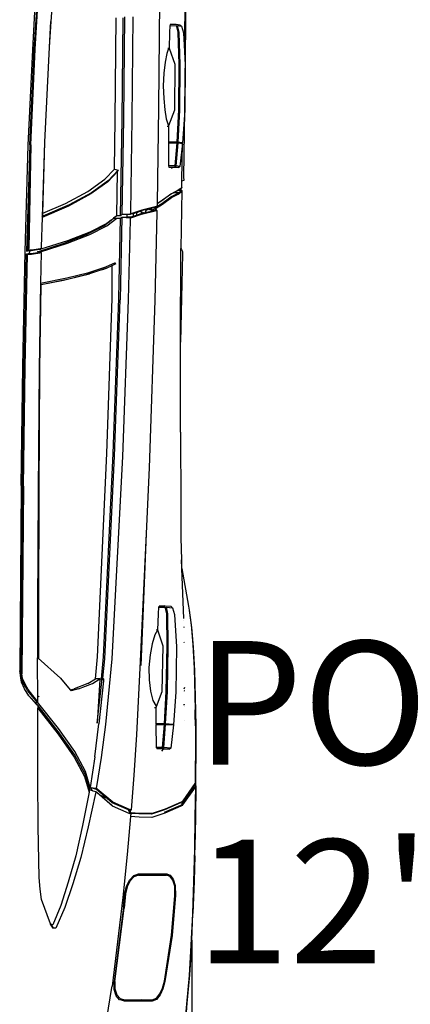
# Model space of a CAD drawing. Units: inches. Extents: x -4737294 to -4736756, y 1716389 to 1717040.
# Tile 10 of 25: x -4737123 to -4737096, y 1716491 to 1716559. Entities that reach past the tile are written whole.
import ezdxf

# ---------------------------------------------------------------- set-up
doc = ezdxf.new("R2010")
doc.units = ezdxf.units.IN
doc.header["$MEASUREMENT"] = 0
doc.layers.add('A-AREA-IDEN', color=250, linetype='Continuous', lineweight=18)
doc.layers.add('A-EQPM-VEHI', color=250, linetype='Continuous', lineweight=13)
doc.layers.add('Edges', color=250, linetype='Continuous')
doc.styles.get("Standard").update_dxf_attribs({"font": 'arial.ttf'})

# ---------------------------------------------------------------- blocks, each defined once
blk = doc.blocks.new('Nissan Qashqai pl')
at = {"layer": 'Edges'}
for p, q in [((10.4889, 12.8119), (10.526, 12.8138)), ((10.4926, 12.8125), (10.5294, 12.8143)), ((10.526, 12.8138), (10.569, 12.8151)), ((10.5294, 12.8143), (10.5719, 12.8156)), ((10.569, 12.8151), (10.5919, 12.8155)), ((10.5719, 12.8156), (10.6176, 12.8164)), ((10.5919, 12.8155), (10.6151, 12.8159)), ((10.5981, 12.8157), (10.5919, 12.8155)), ((10.6174, 12.816), (10.5981, 12.8157)), ((10.6151, 12.8159), (10.6644, 12.8162)), ((10.6176, 12.8164), (10.6651, 12.8167)), ((10.6644, 12.8162), (10.7078, 12.8159)), ((10.6651, 12.8167), (10.666, 12.8167)), ((10.666, 12.8167), (10.677, 12.8167)), ((10.6729, 12.8157), (10.7082, 12.8156)), ((10.6809, 12.8167), (10.677, 12.8167)), ((10.7128, 12.8166), (10.6809, 12.8167)), ((10.7078, 12.8159), (10.7083, 12.8156)), ((10.7082, 12.8156), (10.7078, 12.8159)), ((10.7085, 12.8153), (10.7082, 12.8156)), ((10.7082, 12.8156), (10.7083, 12.8156)), ((10.7083, 12.8156), (10.7087, 12.8153)), ((10.7083, 12.8156), (10.7125, 12.8156)), ((10.7087, 12.8153), (10.7363, 12.7959)), ((10.7139, 12.8164), (10.7125, 12.8156)), ((10.7137, 12.8148), (10.7125, 12.8156)), ((10.7128, 12.8166), (10.7625, 12.8161)), ((10.7128, 12.8166), (10.724, 12.8166)), ((10.7137, 12.8148), (10.7138, 12.8147)), ((10.7418, 12.7947), (10.7138, 12.8147)), ((10.7139, 12.8164), (10.7148, 12.8157)), ((10.7628, 12.8158), (10.7139, 12.8164)), ((10.7148, 12.8157), (10.7429, 12.7956)), ((10.7685, 12.8161), (10.724, 12.8166)), ((10.7625, 12.8161), (10.7628, 12.8161)), ((10.7628, 12.8161), (10.8099, 12.8152)), ((10.8131, 12.8149), (10.7628, 12.8158)), ((10.7688, 12.8161), (10.7685, 12.8161)), ((10.8099, 12.8152), (10.7688, 12.8161)), ((10.8099, 12.8152), (10.8131, 12.8152)), ((10.8134, 12.8152), (10.8131, 12.8152)), ((10.8644, 12.8135), (10.8131, 12.8149)), ((10.8134, 12.8152), (10.8142, 12.8152)), ((10.8142, 12.8152), (10.8142, 12.8152)), ((10.8237, 12.8149), (10.8142, 12.8152)), ((10.8237, 12.8149), (10.864, 12.8138)), ((10.8596, 12.8138), (10.8589, 12.8138)), ((10.8642, 12.8136), (10.8596, 12.8138)), ((10.864, 12.8138), (10.8642, 12.8138)), ((10.8642, 12.8138), (10.9152, 12.812)), ((9.2517, 12.8031), (9.5372, 12.7983)), ((9.641, 12.7991), (9.351, 12.803)), ((9.5176, 12.7972), (9.5372, 12.7983)), ((9.5372, 12.7983), (9.5689, 12.7999)), ((9.5689, 12.7999), (9.641, 12.7991)), ((9.641, 12.7991), (9.6921, 12.7956)), ((9.7466, 12.7978), (9.641, 12.7991)), ((10.3679, 12.7944), (10.4275, 12.8051)), ((10.4275, 12.8051), (10.4304, 12.8056)), ((10.4304, 12.8056), (10.4339, 12.8061)), ((10.4339, 12.8061), (10.4573, 12.8093)), ((10.4339, 12.8061), (10.4345, 12.8062)), ((10.4345, 12.8062), (10.4613, 12.8099)), ((10.4573, 12.8093), (10.4889, 12.8119)), ((10.4613, 12.8099), (10.4926, 12.8125)), ((10.4838, 12.7977), (10.4852, 12.7982)), ((10.5565, 12.7985), (10.5591, 12.7977)), ((10.5615, 12.7978), (10.5617, 12.7985)), ((10.583, 12.7984), (10.5834, 12.798)), ((10.5836, 12.798), (10.5831, 12.7984)), ((10.5847, 12.798), (10.5841, 12.7984)), ((10.5873, 12.7981), (10.5873, 12.7981)), ((10.6087, 12.7983), (10.6087, 12.7984)), ((10.9158, 12.8118), (10.8644, 12.8135)), ((10.9577, 12.8101), (10.9152, 12.812)), ((10.9657, 12.8095), (10.9158, 12.8118)), ((10.9577, 12.8101), (10.9649, 12.8097)), ((10.9577, 12.8101), (11.1283, 12.8101)), ((10.9649, 12.8097), (11.0127, 12.8067)), ((11.0138, 12.8064), (10.9657, 12.8095)), ((11.0127, 12.8067), (11.0576, 12.8026)), ((11.059, 12.8023), (11.0138, 12.8064)), ((11.0576, 12.8026), (11.0798, 12.8008)), ((11.0768, 12.8008), (11.059, 12.8023)), ((9.5052, 12.7918), (9.5044, 12.7856)), ((9.5044, 12.7856), (9.5045, 12.7814)), ((9.5052, 12.7918), (9.5069, 12.7941)), ((9.5061, 12.7878), (9.5069, 12.7941)), ((9.5168, 12.7904), (9.5061, 12.7878)), ((9.5061, 12.7856), (9.5167, 12.7883)), ((9.5063, 12.7755), (9.5061, 12.7856)), ((9.5069, 12.7941), (9.5176, 12.7972)), ((9.5167, 12.7883), (9.5679, 12.7899)), ((9.5679, 12.792), (9.5168, 12.7904)), ((9.5678, 12.7837), (9.5426, 12.7747)), ((9.64, 12.7831), (9.5678, 12.7837)), ((9.6401, 12.7914), (9.5679, 12.792)), ((9.5679, 12.7899), (9.64, 12.7892)), ((9.64, 12.7892), (9.6912, 12.7865)), ((9.6645, 12.7737), (9.64, 12.7831)), ((9.6913, 12.7886), (9.6401, 12.7914)), ((9.6913, 12.7886), (9.6912, 12.7865)), ((9.6912, 12.7865), (9.6912, 12.7811)), ((9.692, 12.7943), (9.6913, 12.7886)), ((9.6921, 12.7956), (9.692, 12.7943)), ((9.6922, 12.7943), (9.692, 12.7943)), ((9.692, 12.7811), (9.6921, 12.7864)), ((9.6922, 12.7943), (9.6921, 12.7956)), ((9.7526, 12.7946), (9.6921, 12.7956)), ((9.6922, 12.7885), (9.6921, 12.7864)), ((9.6921, 12.7864), (9.7288, 12.7832)), ((9.6922, 12.7885), (9.693, 12.7955)), ((9.6922, 12.7885), (9.6922, 12.7943)), ((9.7288, 12.7854), (9.6922, 12.7885)), ((9.693, 12.7955), (9.7296, 12.7914)), ((9.7288, 12.7832), (9.7287, 12.7734)), ((9.7296, 12.7914), (9.7288, 12.7854)), ((9.7306, 12.7834), (9.7288, 12.7854)), ((9.7288, 12.7854), (9.7288, 12.7832)), ((9.7288, 12.7832), (9.7306, 12.7834)), ((9.7296, 12.7914), (9.7314, 12.7895)), ((9.7305, 12.7738), (9.7306, 12.7834)), ((9.7306, 12.7834), (9.7314, 12.7895)), ((9.7314, 12.7895), (9.7313, 12.7798)), ((9.7511, 12.7979), (9.7466, 12.7978)), ((9.7526, 12.7946), (9.7511, 12.7979)), ((9.7623, 12.7945), (9.7526, 12.7946)), ((9.7623, 12.7945), (9.7643, 12.7937)), ((9.7643, 12.7937), (9.7652, 12.7927)), ((9.7643, 12.7937), (9.7648, 12.7929)), ((9.7648, 12.7929), (9.7648, 12.7929)), ((9.7648, 12.7929), (9.7664, 12.7902)), ((9.7652, 12.7927), (9.7665, 12.7907)), ((9.7665, 12.7904), (9.7664, 12.7902)), ((9.7664, 12.7902), (9.7674, 12.7885)), ((9.7667, 12.7933), (9.7665, 12.7907)), ((9.7665, 12.7907), (9.7676, 12.7889)), ((9.7677, 12.7944), (9.7667, 12.7933)), ((9.7676, 12.7931), (9.7667, 12.7933)), ((9.7673, 12.7899), (9.7676, 12.7931)), ((9.7673, 12.7897), (9.7673, 12.7899)), ((9.7673, 12.7897), (9.7676, 12.7889)), ((9.7674, 12.7885), (9.7728, 12.7781)), ((9.769, 12.7926), (9.7676, 12.7931)), ((9.7676, 12.7889), (9.7684, 12.7875)), ((9.7676, 12.7887), (9.7678, 12.7882)), ((9.7677, 12.7944), (9.7677, 12.7944)), ((9.77, 12.7936), (9.7677, 12.7944)), ((9.7677, 12.7944), (9.8598, 12.7928)), ((9.7684, 12.7875), (9.7717, 12.781)), ((9.7712, 12.7892), (9.769, 12.7926)), ((9.7734, 12.7884), (9.77, 12.7936)), ((9.7707, 12.7848), (9.7709, 12.7893)), ((9.7717, 12.781), (9.7707, 12.7848)), ((9.7709, 12.7893), (9.7712, 12.7892)), ((9.7724, 12.7874), (9.7712, 12.7892)), ((9.7778, 12.777), (9.7724, 12.7874)), ((9.7788, 12.778), (9.7734, 12.7884)), ((9.8598, 12.7928), (9.8614, 12.7937)), ((9.8643, 12.7927), (9.8598, 12.7928)), ((9.8614, 12.7937), (9.8647, 12.7956)), ((10.0085, 12.7922), (9.8643, 12.7927)), ((9.8647, 12.7956), (9.869, 12.7954)), ((9.869, 12.7954), (10.0085, 12.7922)), ((10.0124, 12.7922), (10.0085, 12.7922)), ((10.1513, 12.7924), (10.0124, 12.7922)), ((10.1513, 12.7924), (10.2677, 12.793)), ((10.2677, 12.793), (10.3189, 12.7931)), ((10.3189, 12.7931), (10.3537, 12.7939)), ((10.3537, 12.7939), (10.3832, 12.7945)), ((10.3679, 12.7944), (10.3537, 12.7939)), ((10.4468, 12.7976), (10.3679, 12.7944)), ((10.4299, 12.7798), (10.4406, 12.7829)), ((10.4406, 12.7829), (10.4919, 12.7858)), ((10.4503, 12.7976), (10.4502, 12.7976)), ((10.4603, 12.7976), (10.4613, 12.7978)), ((10.4919, 12.7858), (10.564, 12.7851)), ((10.564, 12.7851), (10.6151, 12.7813)), ((10.7363, 12.7959), (10.7376, 12.795)), ((10.7387, 12.794), (10.7376, 12.795)), ((10.7376, 12.795), (10.7378, 12.7946)), ((10.7378, 12.7946), (10.7379, 12.7945)), ((10.7378, 12.7946), (10.7385, 12.7932)), ((10.7385, 12.7932), (10.7497, 12.7679)), ((10.7387, 12.794), (10.7396, 12.7922)), ((10.7396, 12.7922), (10.7507, 12.7669)), ((10.743, 12.7939), (10.7418, 12.7947)), ((10.7432, 12.7954), (10.7426, 12.7954)), ((10.7429, 12.7956), (10.7432, 12.7954)), ((10.7434, 12.793), (10.743, 12.7939)), ((10.7441, 12.7954), (10.7432, 12.7954)), ((10.7432, 12.7954), (10.744, 12.7948)), ((10.7437, 12.7921), (10.7434, 12.793)), ((10.7438, 12.7921), (10.7437, 12.7921)), ((10.7438, 12.7921), (10.7549, 12.7666)), ((10.744, 12.7948), (10.7448, 12.793)), ((10.7448, 12.793), (10.7559, 12.7674)), ((10.8607, 12.7808), (10.8708, 12.7841)), ((10.8716, 12.7832), (10.8622, 12.7801)), ((10.8708, 12.7841), (10.8869, 12.7844)), ((10.887, 12.7835), (10.8716, 12.7832)), ((10.8869, 12.7844), (10.9499, 12.7789)), ((10.9498, 12.7781), (10.887, 12.7835)), ((9.5037, 12.7806), (9.5045, 12.7814)), ((9.5045, 12.7814), (9.5045, 12.7759)), ((9.5045, 12.7759), (9.5063, 12.7755)), ((9.5063, 12.7755), (9.5168, 12.7751)), ((9.5168, 12.7751), (9.5423, 12.7746)), ((9.5423, 12.7746), (9.5422, 12.7736)), ((9.5422, 12.7736), (9.5422, 12.7725)), ((9.5422, 12.7736), (9.5424, 12.7735)), ((9.5426, 12.7747), (9.5423, 12.7746)), ((9.5426, 12.7747), (9.5424, 12.7735)), ((9.5424, 12.7735), (9.5503, 12.7706)), ((9.5503, 12.7706), (9.5641, 12.7681)), ((9.5641, 12.7681), (9.5818, 12.766)), ((9.6215, 12.766), (9.6395, 12.7676)), ((9.6395, 12.7676), (9.654, 12.7697)), ((9.654, 12.7697), (9.6633, 12.7726)), ((9.6633, 12.7726), (9.6645, 12.7737)), ((9.6655, 12.7733), (9.6645, 12.7737)), ((9.6655, 12.7733), (9.6911, 12.7732)), ((9.6655, 12.7713), (9.6655, 12.7733)), ((9.6912, 12.7811), (9.6911, 12.7796)), ((9.6911, 12.7796), (9.6911, 12.7732)), ((9.6911, 12.7732), (9.692, 12.7733)), ((9.692, 12.7811), (9.6912, 12.7811)), ((9.692, 12.7796), (9.692, 12.7811)), ((9.692, 12.7733), (9.692, 12.7796)), ((9.692, 12.7733), (9.7287, 12.7734)), ((9.7287, 12.7734), (9.7305, 12.7738)), ((9.7305, 12.7738), (9.7313, 12.7798)), ((9.733, 12.7782), (9.7313, 12.7798)), ((9.7717, 12.781), (9.7738, 12.7771)), ((9.7728, 12.7781), (9.7832, 12.7637)), ((9.7738, 12.7771), (9.7842, 12.7627)), ((9.7883, 12.7626), (9.7778, 12.777)), ((9.7894, 12.7636), (9.7788, 12.778)), ((10.4263, 12.7665), (10.4274, 12.7674)), ((10.4282, 12.7775), (10.4274, 12.7679)), ((10.4274, 12.7679), (10.4274, 12.7674)), ((10.4274, 12.7674), (10.4275, 12.7586)), ((10.4282, 12.7775), (10.4299, 12.7798)), ((10.4291, 12.77), (10.4299, 12.7798)), ((10.4398, 12.7724), (10.4291, 12.77)), ((10.4291, 12.7677), (10.4398, 12.7701)), ((10.4293, 12.7579), (10.4291, 12.7677)), ((10.4909, 12.773), (10.4398, 12.7724)), ((10.4398, 12.7701), (10.4909, 12.7708)), ((10.5631, 12.7715), (10.4909, 12.773)), ((10.4909, 12.7708), (10.563, 12.7692)), ((10.563, 12.7692), (10.6142, 12.7663)), ((10.6142, 12.7686), (10.5631, 12.7715)), ((10.615, 12.7803), (10.6142, 12.7686)), ((10.6142, 12.7686), (10.6142, 12.7677)), ((10.6142, 12.7677), (10.615, 12.7676)), ((10.6142, 12.7677), (10.6142, 12.7663)), ((10.6151, 12.7813), (10.615, 12.7803)), ((10.615, 12.7676), (10.6151, 12.7803)), ((10.6151, 12.7803), (10.615, 12.7803)), ((10.6151, 12.7676), (10.615, 12.7676)), ((10.6151, 12.7803), (10.6151, 12.7813)), ((10.6151, 12.7685), (10.616, 12.7812)), ((10.6518, 12.7657), (10.6151, 12.7685)), ((10.6151, 12.7676), (10.6151, 12.7685)), ((10.6151, 12.7662), (10.6151, 12.7676)), ((10.616, 12.7812), (10.6526, 12.7768)), ((10.6526, 12.7768), (10.6518, 12.7657)), ((10.6526, 12.7768), (10.6543, 12.7749)), ((10.6537, 12.7658), (10.6543, 12.7749)), ((10.6543, 12.7749), (10.6543, 12.7656)), ((10.7497, 12.7679), (10.7565, 12.7473)), ((10.7507, 12.7669), (10.7575, 12.7462)), ((10.7559, 12.7674), (10.7626, 12.7467)), ((10.8523, 12.7704), (10.8546, 12.7762)), ((10.8523, 12.7255), (10.8523, 12.7704)), ((10.8543, 12.7702), (10.8538, 12.753)), ((10.8565, 12.7757), (10.8543, 12.7702)), ((10.8543, 12.7255), (10.8543, 12.7702)), ((10.8546, 12.7762), (10.8607, 12.7808)), ((10.8622, 12.7801), (10.8565, 12.7757)), ((11.0226, 12.7668), (10.9498, 12.7781)), ((10.9499, 12.7789), (11.0229, 12.7676)), ((11.0339, 12.7639), (11.0226, 12.7668)), ((11.0229, 12.7676), (11.0348, 12.7645)), ((9.4673, 12.7589), (9.6358, 12.7575)), ((9.5818, 12.766), (9.6016, 12.7651)), ((9.6016, 12.7651), (9.6215, 12.766)), ((9.6358, 12.7575), (9.7887, 12.7552)), ((9.7832, 12.7637), (9.7887, 12.7552)), ((9.7842, 12.7627), (9.7891, 12.7552)), ((9.7933, 12.7549), (9.7883, 12.7626)), ((9.7887, 12.7552), (9.7891, 12.7552)), ((9.7891, 12.7552), (9.79, 12.7552)), ((9.7965, 12.7526), (9.7894, 12.7636)), ((9.79, 12.7552), (9.7931, 12.7552)), ((9.7931, 12.7552), (9.7934, 12.7535)), ((9.7931, 12.7552), (9.7933, 12.7549)), ((9.7933, 12.7549), (9.7941, 12.7541)), ((9.7934, 12.7535), (9.7938, 12.7538)), ((9.7934, 12.7535), (9.7937, 12.7524)), ((9.7937, 12.7524), (9.7992, 12.7308)), ((9.7941, 12.7541), (9.7943, 12.7535)), ((9.7955, 12.7516), (9.7943, 12.7535)), ((9.7943, 12.7535), (9.7964, 12.7453)), ((9.7963, 12.7523), (9.7955, 12.7516)), ((9.7963, 12.7523), (9.7963, 12.7524)), ((9.7964, 12.7524), (9.7963, 12.7523)), ((9.7992, 12.7476), (9.7963, 12.7523)), ((9.7967, 12.7526), (9.7964, 12.7524)), ((9.7964, 12.7525), (9.7964, 12.7524)), ((9.7964, 12.7524), (9.7996, 12.7475)), ((9.7983, 12.7541), (9.7965, 12.7526)), ((9.7965, 12.7526), (9.7967, 12.7526)), ((9.7977, 12.7535), (9.7967, 12.7526)), ((9.7967, 12.7526), (9.7986, 12.7526)), ((9.7982, 12.754), (9.7977, 12.7535)), ((9.7983, 12.7541), (9.7982, 12.754)), ((9.7986, 12.7526), (9.7982, 12.754)), ((9.7986, 12.7544), (9.7983, 12.7541)), ((9.7993, 12.755), (9.7986, 12.7544)), ((9.7988, 12.7516), (9.7986, 12.7526)), ((9.7998, 12.7477), (9.7988, 12.7516)), ((9.7999, 12.7522), (9.7993, 12.755)), ((9.7993, 12.755), (9.8024, 12.7549)), ((9.8054, 12.7307), (9.7999, 12.7522)), ((9.8024, 12.7549), (9.9426, 12.7518)), ((9.9426, 12.7518), (10.2081, 12.7424)), ((10.4293, 12.7579), (10.4275, 12.7586)), ((10.4398, 12.7573), (10.4293, 12.7579)), ((10.4653, 12.7564), (10.4398, 12.7573)), ((10.4653, 12.7561), (10.4652, 12.7545)), ((10.4908, 12.7648), (10.4653, 12.7564)), ((10.4653, 12.7564), (10.4653, 12.7561)), ((10.4653, 12.7564), (10.4653, 12.7564)), ((10.4653, 12.7564), (10.4653, 12.7561)), ((10.4653, 12.7561), (10.4653, 12.7561)), ((10.4653, 12.7561), (10.4732, 12.7517)), ((10.4732, 12.7517), (10.4871, 12.7474)), ((10.563, 12.7633), (10.4908, 12.7648)), ((10.5867, 12.7545), (10.563, 12.7633)), ((10.5769, 12.7484), (10.5863, 12.7537)), ((10.5863, 12.7537), (10.5867, 12.7545)), ((10.5885, 12.7538), (10.5867, 12.7545)), ((10.5885, 12.751), (10.5885, 12.7538)), ((10.6141, 12.7537), (10.5885, 12.7538)), ((10.6142, 12.766), (10.6141, 12.7537)), ((10.6141, 12.7537), (10.615, 12.7537)), ((10.6142, 12.7663), (10.6142, 12.766)), ((10.615, 12.7537), (10.6151, 12.7659)), ((10.6517, 12.754), (10.615, 12.7537)), ((10.6151, 12.7662), (10.6518, 12.7634)), ((10.6151, 12.7659), (10.6151, 12.7662)), ((10.6518, 12.7634), (10.6517, 12.754)), ((10.6535, 12.7546), (10.6517, 12.754)), ((10.6536, 12.7639), (10.6518, 12.7657)), ((10.6518, 12.7657), (10.6518, 12.7634)), ((10.6518, 12.7634), (10.6536, 12.7639)), ((10.6543, 12.7656), (10.6535, 12.7546)), ((10.6535, 12.7546), (10.6536, 12.7639)), ((10.6536, 12.7639), (10.6537, 12.7658)), ((10.6537, 12.7658), (10.6543, 12.7656)), ((10.6578, 12.7628), (10.6543, 12.7656)), ((10.8528, 12.7503), (10.8535, 12.7521)), ((10.8535, 12.7521), (10.8538, 12.753)), ((10.8538, 12.7521), (10.8535, 12.7521)), ((10.8538, 12.753), (10.8538, 12.7521)), ((10.8538, 12.7521), (10.8538, 12.7502)), ((11.0429, 12.7597), (11.0339, 12.7639)), ((11.0348, 12.7645), (11.0444, 12.7601)), ((11.0497, 12.7542), (11.0429, 12.7597)), ((11.0444, 12.7601), (11.0516, 12.7542)), ((11.0523, 12.7475), (11.0497, 12.7542)), ((11.0516, 12.7542), (11.0543, 12.7473)), ((9.7964, 12.7453), (9.7992, 12.7476)), ((9.7964, 12.7453), (9.7973, 12.7418)), ((9.7977, 12.7431), (9.7973, 12.7418)), ((9.7973, 12.7418), (9.7977, 12.7409)), ((9.7973, 12.7418), (9.7977, 12.7399)), ((9.7977, 12.7444), (9.7985, 12.7451)), ((9.7985, 12.7451), (9.7977, 12.7431)), ((9.7977, 12.7431), (9.7977, 12.7444)), ((9.7977, 12.7399), (9.7977, 12.7409)), ((9.7977, 12.7409), (9.7987, 12.7388)), ((9.7977, 12.7399), (9.7978, 12.7397)), ((9.7987, 12.7388), (9.7978, 12.7397)), ((9.7978, 12.7397), (9.7987, 12.7362)), ((9.7989, 12.7461), (9.7985, 12.7451)), ((9.7987, 12.7388), (9.7992, 12.7377)), ((9.7987, 12.7362), (9.7992, 12.7377)), ((9.7987, 12.7362), (9.8002, 12.7301)), ((9.7998, 12.7466), (9.7989, 12.7461)), ((9.7998, 12.7466), (9.7992, 12.7476)), ((9.7992, 12.7377), (9.8027, 12.7364)), ((9.7996, 12.7475), (9.7998, 12.7477)), ((9.8002, 12.7461), (9.7996, 12.7475)), ((9.8001, 12.7468), (9.7996, 12.7475)), ((9.8001, 12.7468), (9.7998, 12.7477)), ((9.8003, 12.7458), (9.7998, 12.7466)), ((9.8002, 12.7461), (9.8001, 12.7468)), ((9.8003, 12.7458), (9.8002, 12.7461)), ((9.8027, 12.7364), (9.8003, 12.7458)), ((9.8031, 12.7349), (9.8027, 12.7364)), ((10.2081, 12.7424), (10.312, 12.7377)), ((10.312, 12.7377), (10.5214, 12.7293)), ((10.312, 12.7377), (10.5147, 12.7285)), ((10.4871, 12.7474), (10.5048, 12.744)), ((10.5048, 12.744), (10.5246, 12.7423)), ((10.5246, 12.7423), (10.5445, 12.7425)), ((10.5445, 12.7425), (10.5625, 12.7446)), ((10.5625, 12.7446), (10.5769, 12.7484)), ((10.7565, 12.7473), (10.7563, 12.7273)), ((10.7575, 12.7462), (10.7572, 12.7263)), ((10.7626, 12.7467), (10.7623, 12.7269)), ((10.8528, 12.742), (10.8528, 12.7503)), ((10.8528, 12.742), (10.8538, 12.742)), ((10.8528, 12.7419), (10.8528, 12.742)), ((10.8538, 12.7419), (10.8528, 12.7419)), ((10.8528, 12.7242), (10.8528, 12.7419)), ((10.8538, 12.7502), (10.8538, 12.742)), ((10.8538, 12.742), (10.8538, 12.7419)), ((10.8538, 12.7214), (10.8538, 12.7419)), ((11.0528, 12.73), (11.0523, 12.7475)), ((11.0523, 12.7312), (11.0523, 12.7475)), ((11.0543, 12.7473), (11.0543, 12.7035)), ((9.7992, 12.7308), (9.8044, 12.7151)), ((9.8002, 12.7301), (9.8008, 12.7285)), ((9.8008, 12.7285), (9.8014, 12.7303)), ((9.8008, 12.7285), (9.8014, 12.7265)), ((9.8014, 12.7303), (9.8031, 12.7349)), ((9.8043, 12.7303), (9.8014, 12.7303)), ((9.8014, 12.7265), (9.803, 12.723)), ((9.8014, 12.7265), (9.8026, 12.723)), ((9.803, 12.723), (9.8026, 12.723)), ((9.8026, 12.723), (9.8046, 12.7171)), ((9.8067, 12.7229), (9.803, 12.723)), ((9.8043, 12.7303), (9.8031, 12.7349)), ((9.8044, 12.73), (9.8043, 12.7303)), ((9.8067, 12.7229), (9.8044, 12.73)), ((9.8106, 12.715), (9.8054, 12.7307)), ((9.8086, 12.7171), (9.8067, 12.7229)), ((10.5147, 12.7285), (10.6318, 12.7228)), ((10.6318, 12.7228), (10.6955, 12.7184)), ((10.7563, 12.7273), (10.7553, 12.7134)), ((10.7572, 12.7263), (10.7563, 12.7126)), ((10.7623, 12.7269), (10.7615, 12.7131)), ((10.8528, 12.7242), (10.8523, 12.7255)), ((10.8538, 12.7214), (10.8528, 12.7242)), ((10.855, 12.7181), (10.8538, 12.7214)), ((10.8543, 12.7255), (10.8569, 12.7184)), ((11.0523, 12.7312), (11.0528, 12.73)), ((11.0523, 12.7287), (11.0523, 12.7312)), ((11.0528, 12.7274), (11.0523, 12.7287)), ((11.0523, 12.7037), (11.0523, 12.7287)), ((11.0528, 12.7274), (11.0528, 12.73)), ((11.0528, 12.73), (11.0538, 12.7273)), ((11.0528, 12.7274), (11.0528, 12.6985)), ((11.0538, 12.7273), (11.0538, 12.7018)), ((9.6538, 12.7157), (9.4919, 12.7173)), ((9.802, 12.7133), (9.6538, 12.7157)), ((9.8051, 12.7132), (9.802, 12.7133)), ((9.8044, 12.7151), (9.8051, 12.7132)), ((9.8046, 12.7171), (9.8086, 12.7171)), ((9.8046, 12.7171), (9.8055, 12.7143)), ((9.8061, 12.6994), (9.8051, 12.7132)), ((9.8055, 12.7143), (9.8058, 12.7073)), ((9.8058, 12.7073), (9.8098, 12.7073)), ((9.8058, 12.7073), (9.8061, 12.6994)), ((9.8096, 12.7142), (9.8086, 12.7171)), ((9.8098, 12.7073), (9.8096, 12.7142)), ((9.8101, 12.6993), (9.8098, 12.7073)), ((9.8101, 12.6993), (9.8112, 12.7131)), ((9.8112, 12.7131), (9.8106, 12.715)), ((9.8143, 12.713), (9.8112, 12.7131)), ((9.9414, 12.71), (9.8143, 12.713)), ((10.19, 12.7008), (9.9414, 12.71)), ((10.6955, 12.7184), (10.7509, 12.714)), ((10.7501, 12.7114), (10.7387, 12.6849)), ((10.7507, 12.7098), (10.7397, 12.684)), ((10.7563, 12.7109), (10.7449, 12.6843)), ((10.7507, 12.7132), (10.7501, 12.7114)), ((10.7506, 12.7111), (10.7507, 12.7132)), ((10.7507, 12.7132), (10.7509, 12.714)), ((10.751, 12.7132), (10.7507, 12.7132)), ((10.7511, 12.7107), (10.7507, 12.7098)), ((10.7524, 12.7106), (10.7507, 12.7098)), ((10.7522, 12.7131), (10.7509, 12.714)), ((10.7516, 12.7131), (10.7509, 12.714)), ((10.7519, 12.7128), (10.7511, 12.7107)), ((10.7522, 12.7131), (10.7516, 12.7131)), ((10.7519, 12.7128), (10.7516, 12.7131)), ((10.7526, 12.7124), (10.7519, 12.7128)), ((10.7553, 12.7134), (10.7522, 12.7131)), ((10.7524, 12.7106), (10.7526, 12.7124)), ((10.7556, 12.7122), (10.7524, 12.7106)), ((10.7526, 12.7124), (10.7526, 12.7127)), ((10.7532, 12.712), (10.7526, 12.7124)), ((10.7556, 12.7122), (10.7532, 12.712)), ((10.7561, 12.7125), (10.7556, 12.7122)), ((10.7561, 12.7125), (10.7563, 12.7126)), ((10.7563, 12.7125), (10.7561, 12.7125)), ((10.7563, 12.7123), (10.7561, 12.7123)), ((10.7563, 12.7126), (10.7573, 12.7135)), ((10.7563, 12.7126), (10.7563, 12.7125)), ((10.7569, 12.7125), (10.7563, 12.7109)), ((10.7569, 12.7125), (10.7563, 12.7125)), ((10.7563, 12.7125), (10.7563, 12.7123)), ((10.7573, 12.7135), (10.7569, 12.7125)), ((10.7573, 12.7135), (10.7604, 12.7132)), ((10.7604, 12.7132), (10.7615, 12.7131)), ((10.7615, 12.7131), (10.8218, 12.7077)), ((10.8218, 12.7077), (10.8896, 12.7008)), ((10.8622, 12.7114), (10.855, 12.7181)), ((10.8569, 12.7184), (10.8637, 12.712)), ((10.8718, 12.7068), (10.8622, 12.7114)), ((10.8637, 12.712), (10.8727, 12.7077)), ((10.8836, 12.7041), (10.8718, 12.7068)), ((10.8727, 12.7077), (10.8839, 12.7051)), ((10.8839, 12.7051), (10.9067, 12.7029)), ((9.4922, 12.7033), (9.654, 12.7018)), ((9.6552, 12.6997), (9.4936, 12.7013)), ((9.6552, 12.6888), (9.4936, 12.6904)), ((9.654, 12.7018), (9.8061, 12.6994)), ((9.8078, 12.6971), (9.6552, 12.6997)), ((9.7337, 12.6875), (9.6552, 12.6888)), ((9.7337, 12.6875), (9.7357, 12.6935)), ((9.7357, 12.6935), (9.7378, 12.6924)), ((9.7357, 12.6935), (9.7519, 12.678)), ((9.7378, 12.6924), (9.754, 12.677)), ((9.8078, 12.6913), (9.7378, 12.6924)), ((9.8061, 12.6994), (9.8078, 12.6971)), ((9.8078, 12.6971), (9.8078, 12.6913)), ((9.8078, 12.6913), (9.8119, 12.6862)), ((9.8119, 12.697), (9.8101, 12.6993)), ((9.8101, 12.6993), (9.9411, 12.6966)), ((9.9393, 12.6944), (9.8119, 12.697)), ((9.8119, 12.6912), (9.8119, 12.697)), ((9.8241, 12.6756), (9.8119, 12.6912)), ((9.8119, 12.6862), (9.8119, 12.6912)), ((9.8891, 12.6741), (9.8818, 12.6891)), ((9.8867, 12.6842), (9.8838, 12.6901)), ((10.1849, 12.6857), (9.9393, 12.6944)), ((10.1894, 12.6879), (9.9411, 12.6966)), ((10.5113, 12.6839), (10.19, 12.7008)), ((10.9054, 12.702), (10.8836, 12.7041)), ((10.8896, 12.7008), (11.0304, 12.6838)), ((10.9054, 12.702), (11.0232, 12.6871)), ((11.0231, 12.6882), (10.9067, 12.7029)), ((11.035, 12.6883), (11.0443, 12.6911)), ((11.0458, 12.6903), (11.0358, 12.6872)), ((11.0443, 12.6911), (11.0501, 12.6964)), ((11.052, 12.6958), (11.0458, 12.6903)), ((11.0501, 12.6964), (11.0523, 12.7037)), ((11.0528, 12.6985), (11.052, 12.6958)), ((11.0538, 12.7018), (11.0528, 12.6985)), ((11.0543, 12.7035), (11.0538, 12.7018)), ((9.7499, 12.6721), (9.7337, 12.6875)), ((9.7519, 12.678), (9.7713, 12.6512)), ((9.754, 12.677), (9.7733, 12.6502)), ((9.8147, 12.6826), (9.8119, 12.6862)), ((9.8147, 12.6826), (9.8147, 12.6826)), ((9.8147, 12.6826), (9.8201, 12.6756)), ((9.8241, 12.6706), (9.8147, 12.6826)), ((9.8201, 12.6756), (9.8338, 12.6486)), ((9.8378, 12.6485), (9.8241, 12.6756)), ((9.9393, 12.684), (9.8867, 12.6842)), ((9.8911, 12.675), (9.8867, 12.6842)), ((9.8978, 12.6472), (9.8891, 12.6741)), ((9.8911, 12.6749), (9.8911, 12.675)), ((9.8931, 12.6691), (9.8911, 12.6749)), ((9.8911, 12.6749), (9.8998, 12.6481)), ((10.1849, 12.6754), (9.9393, 12.684)), ((10.5079, 12.6703), (10.1849, 12.6857)), ((10.5079, 12.6607), (10.1849, 12.6754)), ((10.5109, 12.6721), (10.1894, 12.6879)), ((10.6152, 12.674), (10.5113, 12.6839)), ((10.6678, 12.6672), (10.6152, 12.674)), ((10.7387, 12.6849), (10.7177, 12.6604)), ((10.7334, 12.6766), (10.7186, 12.6593)), ((10.7449, 12.6843), (10.7232, 12.6594)), ((10.7438, 12.6836), (10.7265, 12.6635)), ((10.7265, 12.6635), (10.7316, 12.6741)), ((10.7397, 12.684), (10.7334, 12.6766)), ((11.0231, 12.6882), (11.035, 12.6883)), ((11.0358, 12.6872), (11.0232, 12.6871)), ((11.0357, 12.6829), (11.0304, 12.6838)), ((11.0491, 12.6807), (11.0357, 12.6829)), ((11.0449, 12.6812), (11.0448, 12.6812)), ((11.0492, 12.6807), (11.0491, 12.6807)), ((11.1336, 12.667), (11.0492, 12.6807)), ((9.7692, 12.6453), (9.7499, 12.6721)), ((9.8378, 12.6435), (9.8241, 12.6706)), ((9.8931, 12.669), (9.8931, 12.6691)), ((9.8931, 12.669), (9.9018, 12.6421)), ((10.543, 12.6671), (10.5079, 12.6703)), ((10.543, 12.6576), (10.5079, 12.6607)), ((10.5417, 12.6693), (10.5109, 12.6721)), ((10.5417, 12.6693), (10.5427, 12.6702)), ((10.5417, 12.6693), (10.543, 12.6671)), ((10.5436, 12.6687), (10.5427, 12.6702)), ((10.5427, 12.6702), (10.5458, 12.67)), ((10.544, 12.6678), (10.543, 12.6671)), ((10.543, 12.6646), (10.543, 12.6671)), ((10.543, 12.6646), (10.543, 12.6576)), ((10.5439, 12.6646), (10.543, 12.6646)), ((10.5502, 12.6526), (10.543, 12.6646)), ((10.5502, 12.6456), (10.543, 12.6576)), ((10.544, 12.6678), (10.5436, 12.6687)), ((10.5439, 12.6646), (10.613, 12.6601)), ((10.547, 12.6674), (10.544, 12.6678)), ((10.5458, 12.67), (10.6144, 12.6629)), ((10.613, 12.6601), (10.547, 12.6674)), ((10.6664, 12.6566), (10.6144, 12.6629)), ((10.7137, 12.6595), (10.6678, 12.6672)), ((10.7165, 12.6591), (10.7137, 12.6595)), ((10.7186, 12.6593), (10.7155, 12.649)), ((10.7155, 12.649), (10.7165, 12.6591)), ((10.7177, 12.6604), (10.7165, 12.6591)), ((10.7221, 12.6581), (10.7209, 12.654)), ((10.7232, 12.6594), (10.7221, 12.6581)), ((10.7221, 12.6581), (10.7224, 12.6587)), ((10.7221, 12.6581), (10.7247, 12.6575)), ((10.7265, 12.6635), (10.7224, 12.6587)), ((10.7247, 12.6575), (10.7776, 12.646)), ((9.7885, 12.6099), (9.7692, 12.6453)), ((9.7713, 12.6512), (9.7905, 12.6158)), ((9.7733, 12.6502), (9.7925, 12.6148)), ((9.8338, 12.6486), (9.8475, 12.613)), ((9.8516, 12.6129), (9.8378, 12.6485)), ((9.8516, 12.6079), (9.8378, 12.6435)), ((9.9066, 12.6119), (9.8978, 12.6472)), ((9.9086, 12.6129), (9.8998, 12.6481)), ((9.9018, 12.6421), (9.9106, 12.6068)), ((10.5584, 12.6306), (10.5502, 12.6526)), ((10.5502, 12.6456), (10.5584, 12.6236)), ((10.6664, 12.6566), (10.7155, 12.649)), ((10.7155, 12.649), (10.69, 12.6414)), ((10.7155, 12.6473), (10.6943, 12.641)), ((10.6976, 12.6401), (10.7228, 12.6477)), ((10.7209, 12.654), (10.7155, 12.6485)), ((10.7155, 12.649), (10.7155, 12.6485)), ((10.7155, 12.6485), (10.7155, 12.6473)), ((10.7192, 12.6484), (10.7155, 12.6473)), ((10.7209, 12.654), (10.7192, 12.6484)), ((10.7228, 12.6477), (10.7192, 12.6484)), ((10.7228, 12.6477), (10.7754, 12.637)), ((10.7776, 12.646), (10.8264, 12.6341)), ((10.5584, 12.6306), (10.5617, 12.619)), ((10.69, 12.6414), (10.6583, 12.6245)), ((10.6943, 12.641), (10.6627, 12.6241)), ((10.6671, 12.6238), (10.6976, 12.6401)), ((10.7754, 12.637), (10.8239, 12.6261)), ((10.8264, 12.6341), (10.8682, 12.6216)), ((9.7905, 12.6158), (9.8087, 12.574)), ((9.7925, 12.6148), (9.8107, 12.573)), ((9.8475, 12.613), (9.8611, 12.5708)), ((9.8652, 12.5704), (9.8516, 12.6129)), ((9.9149, 12.5705), (9.9066, 12.6119)), ((9.9169, 12.5714), (9.9086, 12.6129)), ((10.5419, 12.6018), (10.56, 12.6176)), ((10.56, 12.6176), (10.5584, 12.6236)), ((10.56, 12.6176), (10.5617, 12.619)), ((10.6583, 12.6245), (10.6215, 12.5986)), ((10.6627, 12.6241), (10.6261, 12.5984)), ((10.6306, 12.5982), (10.6671, 12.6238)), ((10.8239, 12.6261), (10.8653, 12.6144)), ((10.8653, 12.6144), (10.9026, 12.6025)), ((10.8682, 12.6216), (10.9059, 12.6087)), ((9.8039, 12.5741), (9.7885, 12.6099)), ((9.8652, 12.5654), (9.8516, 12.6079)), ((9.9106, 12.6068), (9.9177, 12.5714)), ((10.51, 12.5666), (10.5419, 12.6018)), ((10.6215, 12.5986), (10.5796, 12.5655)), ((10.5892, 12.5659), (10.6306, 12.5982)), ((10.6261, 12.5984), (10.593, 12.5726)), ((10.9026, 12.6025), (10.933, 12.5901)), ((10.9059, 12.6087), (10.9384, 12.5945)), ((9.471, 12.5888), (9.4997, 12.5869)), ((9.5404, 12.5844), (9.4997, 12.5869)), ((9.4997, 12.5869), (9.5403, 12.5842)), ((9.5403, 12.5842), (9.6913, 12.5767)), ((9.6912, 12.5774), (9.5404, 12.5844)), ((10.9316, 12.586), (10.8932, 12.572)), ((10.9316, 12.586), (10.9334, 12.5872)), ((10.932, 12.5862), (10.9316, 12.586)), ((10.9335, 12.5871), (10.932, 12.5862)), ((10.933, 12.5901), (10.9334, 12.5872)), ((10.9334, 12.5872), (10.9386, 12.5905)), ((10.9334, 12.5872), (10.9335, 12.5871)), ((10.9386, 12.5905), (10.9335, 12.5871)), ((10.9384, 12.5945), (10.9386, 12.5905)), ((9.5437, 12.5619), (9.4735, 12.5663)), ((9.5438, 12.5605), (9.4736, 12.5648)), ((9.8039, 12.5741), (9.6912, 12.5774)), ((9.6913, 12.5767), (9.8099, 12.573)), ((9.8087, 12.574), (9.8039, 12.5741)), ((9.8099, 12.573), (9.8087, 12.574)), ((9.8099, 12.573), (9.8107, 12.573)), ((9.8107, 12.573), (9.8573, 12.5716)), ((9.8573, 12.5716), (9.8603, 12.5715)), ((9.8603, 12.5715), (9.8605, 12.5696)), ((9.8611, 12.5708), (9.8603, 12.5715)), ((9.8605, 12.5696), (9.8626, 12.5564)), ((9.8612, 12.5707), (9.8611, 12.5708)), ((9.8612, 12.5707), (9.8615, 12.5688)), ((9.8615, 12.5688), (9.8635, 12.5556)), ((9.8652, 12.5706), (9.8664, 12.5714)), ((9.8652, 12.5706), (9.8665, 12.5695)), ((9.8652, 12.5704), (9.8652, 12.5706)), ((9.8652, 12.5704), (9.8652, 12.5704)), ((9.8652, 12.5704), (9.8652, 12.5654)), ((9.8655, 12.5687), (9.8652, 12.5704)), ((9.8675, 12.5555), (9.8655, 12.5687)), ((9.8665, 12.5695), (9.8664, 12.5714)), ((9.8664, 12.5714), (9.9149, 12.5705)), ((9.8686, 12.5562), (9.8665, 12.5695)), ((9.9149, 12.5705), (10.0505, 12.5681)), ((9.9177, 12.5714), (9.9169, 12.5714)), ((10.0501, 12.5695), (9.9177, 12.5714)), ((10.2453, 12.568), (10.0501, 12.5695)), ((10.0505, 12.5681), (10.2453, 12.5664)), ((10.4292, 12.5674), (10.2453, 12.568)), ((10.2453, 12.5664), (10.4289, 12.5658)), ((10.4289, 12.5658), (10.5092, 12.5658)), ((10.5099, 12.5674), (10.4292, 12.5674)), ((10.5099, 12.5674), (10.5092, 12.5658)), ((10.5092, 12.5658), (10.5094, 12.5658)), ((10.5094, 12.5658), (10.51, 12.5666)), ((10.5783, 12.5659), (10.5094, 12.5658)), ((10.51, 12.5666), (10.5099, 12.5674)), ((10.5764, 12.5642), (10.5598, 12.5507)), ((10.5834, 12.5641), (10.57, 12.5517)), ((10.5709, 12.5675), (10.5705, 12.5671)), ((10.5719, 12.5682), (10.5709, 12.5675)), ((10.5783, 12.5659), (10.5764, 12.5642)), ((10.5776, 12.5633), (10.5783, 12.5659)), ((10.5796, 12.5655), (10.5776, 12.5633)), ((10.5796, 12.5655), (10.5783, 12.5659)), ((10.5796, 12.562), (10.5796, 12.5655)), ((10.5838, 12.5653), (10.5821, 12.5633)), ((10.584, 12.5647), (10.5834, 12.5641)), ((10.584, 12.5655), (10.5838, 12.5653)), ((10.593, 12.5726), (10.584, 12.5655)), ((10.584, 12.5655), (10.5841, 12.5655)), ((10.584, 12.5654), (10.584, 12.5655)), ((10.5847, 12.5655), (10.584, 12.5647)), ((10.584, 12.5647), (10.584, 12.5654)), ((10.5851, 12.5659), (10.5841, 12.5655)), ((10.5841, 12.5655), (10.5847, 12.5655)), ((10.5851, 12.5659), (10.5847, 12.5655)), ((10.5851, 12.5659), (10.5892, 12.5659)), ((10.6988, 12.5662), (10.5892, 12.5659)), ((10.7769, 12.5667), (10.6988, 12.5662)), ((10.858, 12.5683), (10.7769, 12.5667)), ((10.8766, 12.5697), (10.858, 12.5683)), ((10.8932, 12.572), (10.8766, 12.5697)), ((9.5443, 12.5579), (9.4739, 12.5621)), ((9.6953, 12.5549), (9.5437, 12.5619)), ((9.6954, 12.5535), (9.5438, 12.5605)), ((9.696, 12.551), (9.5443, 12.5579)), ((9.6953, 12.5549), (9.8598, 12.5517)), ((9.6953, 12.5549), (9.863, 12.5497)), ((9.6954, 12.5535), (9.8641, 12.5483)), ((9.8644, 12.5459), (9.696, 12.551)), ((9.8629, 12.5516), (9.8598, 12.5517)), ((9.8626, 12.5564), (9.8627, 12.5532)), ((9.8637, 12.5532), (9.8627, 12.5532)), ((9.8627, 12.5532), (9.8629, 12.5516)), ((9.8629, 12.5516), (9.863, 12.5497)), ((9.8641, 12.5483), (9.863, 12.5497)), ((9.8635, 12.5556), (9.8637, 12.5532)), ((9.8643, 12.5532), (9.8637, 12.5532)), ((9.8637, 12.5532), (9.8638, 12.5508)), ((9.8638, 12.5508), (9.8641, 12.5483)), ((9.8677, 12.5531), (9.8643, 12.5532)), ((9.8677, 12.5531), (9.8675, 12.5555)), ((9.8678, 12.5507), (9.8677, 12.5531)), ((9.8681, 12.5482), (9.8678, 12.5507)), ((9.8681, 12.5482), (9.869, 12.5496)), ((10.0476, 12.5445), (9.8681, 12.5482)), ((9.8689, 12.5515), (9.8686, 12.5562)), ((9.869, 12.5496), (9.8689, 12.5515)), ((10.0477, 12.5459), (9.869, 12.5496)), ((10.5598, 12.5507), (10.5522, 12.5465)), ((10.5583, 12.5481), (10.5546, 12.546)), ((10.5551, 12.5457), (10.5583, 12.5481)), ((10.5612, 12.5498), (10.5583, 12.5481)), ((10.57, 12.5517), (10.5589, 12.5451)), ((10.5776, 12.5633), (10.5612, 12.5498)), ((10.57, 12.5517), (10.5821, 12.5633)), ((10.0472, 12.5423), (9.8644, 12.5459)), ((10.2357, 12.5398), (10.0472, 12.5423)), ((10.2367, 12.5419), (10.0476, 12.5445)), ((10.2369, 12.5433), (10.0477, 12.5459)), ((10.2357, 12.5398), (10.53, 12.5373)), ((10.2367, 12.5419), (10.5351, 12.5392)), ((10.2369, 12.5433), (10.5348, 12.5406)), ((10.4153, 12.5384), (10.4176, 12.5384)), ((10.4176, 12.5384), (10.4181, 12.5384)), ((10.4181, 12.5384), (10.4552, 12.538)), ((10.4181, 12.5384), (10.4181, 12.5384)), ((10.4778, 12.5378), (10.53, 12.5373)), ((10.5301, 12.5373), (10.53, 12.5373)), ((10.5335, 12.5378), (10.5301, 12.5373)), ((10.5419, 12.5391), (10.5335, 12.5378)), ((10.5422, 12.542), (10.5348, 12.5406)), ((10.5418, 12.5405), (10.5351, 12.5392)), ((10.5424, 12.5406), (10.5418, 12.5405)), ((10.5419, 12.5391), (10.5463, 12.541)), ((10.5479, 12.54), (10.5419, 12.5391)), ((10.5522, 12.5465), (10.5422, 12.542)), ((10.5495, 12.5438), (10.5424, 12.5406)), ((10.5463, 12.541), (10.5551, 12.5457)), ((10.5589, 12.5451), (10.5479, 12.54)), ((10.5546, 12.546), (10.5495, 12.5438))]:
    blk.add_line(p, q, dxfattribs=at)
blk = doc.blocks.new('car')
blk.add_blockref('Nissan Qashqai pl', (-9.7433, -11.9151))

msp = doc.modelspace()

# ---------------------------------------------------------------- block references
at = {"layer": 'A-EQPM-VEHI', "xscale": 43.56002006885659, "yscale": 43.56002006885659, "zscale": 43.56002006885659, "rotation": 270}
msp.add_blockref('car', (-4737150.017, 1716548.61), dxfattribs=at)

# ---------------------------------------------------------------- texts
at = {"layer": 'A-AREA-IDEN'}
for s, height, p in [('PORCH', 8.5453, (-4737110.743, 1716507.85)), ('12\'0"X16\'8"', 8.54529, (-4737110.743, 1716494.123))]:
    msp.add_text(s, height=height, dxfattribs=at).set_placement(p)

doc.saveas('drawing.dxf')
